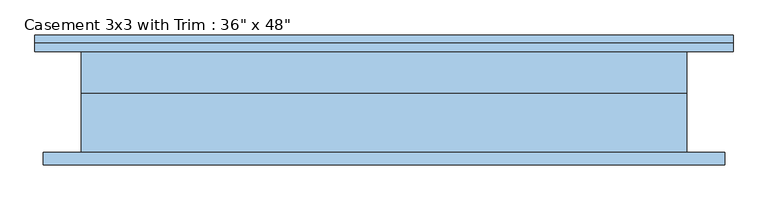
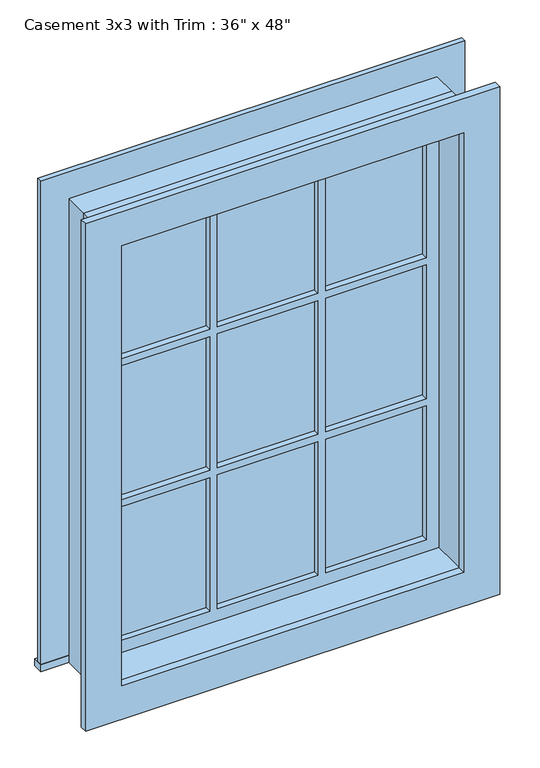
"""IFC4 building model written with IfcOpenShell, lengths in millimetres: window geometry."""

from ifc_helpers import new_model, si_unit, frame, origin, place, context, project, spatial, polyline, outline, extrude, source, transform, mapped, element, save


def window_d6f340c1(model_context):
    return source(origin(), model_context, "Body", "SweptSolid", [
        extrude(outline(polyline([(-527.05, 101.6), (527.05, 101.6), (527.05, 76.2), (-527.05, 76.2), (-527.05, 101.6)])), frame((0.0, 0.0, 1219.2), z_axis=(0.0, 0.0, 1.0), x_axis=(1.0, 0.0, 0.0)), (0.0, 0.0, 1.0), 19.05),
        extrude(outline(polyline([(2419.35, -438.15), (2419.35, 438.15), (1238.25, 438.15), (1238.25, 527.05), (2508.25, 527.05), (2508.25, -527.05), (1238.25, -527.05), (1238.25, -438.15), (2419.35, -438.15)])), frame((0.0, 76.2, 0.0), z_axis=(0.0, 1.0, 0.0), x_axis=(0.0, 0.0, 1.0)), (0.0, 0.0, 1.0), 12.7),
        extrude(outline(polyline([(143.9333333, 41.275), (393.7, 41.275), (393.7, 28.575), (143.9333333, 28.575), (143.9333333, 41.275)])), frame((0.0, 0.0, 2023.5333333), z_axis=(0.0, 0.0, 1.0), x_axis=(1.0, 0.0, 0.0)), (0.0, 0.0, 1.0), 351.3666667),
        extrude(outline(polyline([(-124.8833333, 41.275), (124.8833333, 41.275), (124.8833333, 28.575), (-124.8833333, 28.575), (-124.8833333, 41.275)])), frame((0.0, 0.0, 2023.5333333), z_axis=(0.0, 0.0, 1.0), x_axis=(1.0, 0.0, 0.0)), (0.0, 0.0, 1.0), 351.3666667),
        extrude(outline(polyline([(-393.7, 41.275), (-143.9333333, 41.275), (-143.9333333, 28.575), (-393.7, 28.575), (-393.7, 41.275)])), frame((0.0, 0.0, 2023.5333333), z_axis=(0.0, 0.0, 1.0), x_axis=(1.0, 0.0, 0.0)), (0.0, 0.0, 1.0), 351.3666667),
        extrude(outline(polyline([(-393.7, 41.275), (-143.9333333, 41.275), (-143.9333333, 28.575), (-393.7, 28.575), (-393.7, 41.275)])), frame((0.0, 0.0, 1653.1166667), z_axis=(0.0, 0.0, 1.0), x_axis=(1.0, 0.0, 0.0)), (0.0, 0.0, 1.0), 351.3666667),
        extrude(outline(polyline([(-124.8833333, 41.275), (124.8833333, 41.275), (124.8833333, 28.575), (-124.8833333, 28.575), (-124.8833333, 41.275)])), frame((0.0, 0.0, 1653.1166667), z_axis=(0.0, 0.0, 1.0), x_axis=(1.0, 0.0, 0.0)), (0.0, 0.0, 1.0), 351.3666667),
        extrude(outline(polyline([(143.9333333, 41.275), (393.7, 41.275), (393.7, 28.575), (143.9333333, 28.575), (143.9333333, 41.275)])), frame((0.0, 0.0, 1653.1166667), z_axis=(0.0, 0.0, 1.0), x_axis=(1.0, 0.0, 0.0)), (0.0, 0.0, 1.0), 351.3666667),
        extrude(outline(polyline([(143.9333333, 41.275), (393.7, 41.275), (393.7, 28.575), (143.9333333, 28.575), (143.9333333, 41.275)])), frame((0.0, 0.0, 1282.7), z_axis=(0.0, 0.0, 1.0), x_axis=(1.0, 0.0, 0.0)), (0.0, 0.0, 1.0), 351.3666667),
        extrude(outline(polyline([(-124.8833333, 41.275), (124.8833333, 41.275), (124.8833333, 28.575), (-124.8833333, 28.575), (-124.8833333, 41.275)])), frame((0.0, 0.0, 1282.7), z_axis=(0.0, 0.0, 1.0), x_axis=(1.0, 0.0, 0.0)), (0.0, 0.0, 1.0), 351.3666667),
        extrude(outline(polyline([(-393.7, 41.275), (-143.9333333, 41.275), (-143.9333333, 28.575), (-393.7, 28.575), (-393.7, 41.275)])), frame((0.0, 0.0, 1282.7), z_axis=(0.0, 0.0, 1.0), x_axis=(1.0, 0.0, 0.0)), (0.0, 0.0, 1.0), 351.3666667),
        extrude(outline(polyline([(2495.55, 514.35), (2495.55, -514.35), (1162.05, -514.35), (1162.05, 514.35), (2495.55, 514.35)]), holes=[polyline([(2406.65, 425.45), (1250.95, 425.45), (1250.95, -425.45), (2406.65, -425.45), (2406.65, 425.45)])]), frame((0.0, -95.25, 0.0), z_axis=(0.0, 1.0, 0.0), x_axis=(0.0, 0.0, 1.0)), (0.0, 0.0, 1.0), 19.05),
        extrude(outline(polyline([(2419.35, -438.15), (1238.25, -438.15), (1238.25, 438.15), (2419.35, 438.15), (2419.35, -438.15)]), holes=[polyline([(2374.9, -143.9333333), (2023.5333333, -143.9333333), (2023.5333333, -393.7), (2374.9, -393.7), (2374.9, -143.9333333)]), polyline([(2004.4833333, -143.9333333), (1653.1166667, -143.9333333), (1653.1166667, -393.7), (2004.4833333, -393.7), (2004.4833333, -143.9333333)]), polyline([(1634.0666667, -143.9333333), (1282.7, -143.9333333), (1282.7, -393.7), (1634.0666667, -393.7), (1634.0666667, -143.9333333)]), polyline([(2374.9, 124.8833333), (2023.5333333, 124.8833333), (2023.5333333, -124.8833333), (2374.9, -124.8833333), (2374.9, 124.8833333)]), polyline([(2004.4833333, 124.8833333), (1653.1166667, 124.8833333), (1653.1166667, -124.8833333), (2004.4833333, -124.8833333), (2004.4833333, 124.8833333)]), polyline([(1634.0666667, 124.8833333), (1282.7, 124.8833333), (1282.7, -124.8833333), (1634.0666667, -124.8833333), (1634.0666667, 124.8833333)]), polyline([(2374.9, 393.7), (2023.5333333, 393.7), (2023.5333333, 143.9333333), (2374.9, 143.9333333), (2374.9, 393.7)]), polyline([(2004.4833333, 393.7), (1653.1166667, 393.7), (1653.1166667, 143.9333333), (2004.4833333, 143.9333333), (2004.4833333, 393.7)]), polyline([(1634.0666667, 393.7), (1282.7, 393.7), (1282.7, 143.9333333), (1634.0666667, 143.9333333), (1634.0666667, 393.7)])]), frame((0.0, 12.7, 0.0), z_axis=(0.0, 1.0, 0.0), x_axis=(0.0, 0.0, 1.0)), (0.0, 0.0, 1.0), 44.45),
        extrude(outline(polyline([(2438.4, -457.2), (1219.2, -457.2), (1219.2, 457.2), (2438.4, 457.2), (2438.4, -457.2)]), holes=[polyline([(2406.65, -425.45), (2406.65, 425.45), (1250.95, 425.45), (1250.95, -425.45), (2406.65, -425.45)])]), frame((0.0, -76.2, 0.0), z_axis=(0.0, 1.0, 0.0), x_axis=(0.0, 0.0, 1.0)), (0.0, 0.0, 1.0), 88.9),
        extrude(outline(polyline([(2438.4, 457.2), (2438.4, -457.2), (1219.2, -457.2), (1219.2, 457.2), (2438.4, 457.2)]), holes=[polyline([(2419.35, 438.15), (1238.25, 438.15), (1238.25, -438.15), (2419.35, -438.15), (2419.35, 438.15)])]), frame((0.0, 12.7, 0.0), z_axis=(0.0, 1.0, 0.0), x_axis=(0.0, 0.0, 1.0)), (0.0, 0.0, 1.0), 63.5),
    ])


if __name__ == "__main__":
    model = new_model("IFC4")
    model_context = context("Model", 3, world=origin())
    ifc_project = project(units=[si_unit("LENGTHUNIT", "METRE", prefix="MILLI")], contexts=[model_context])
    site = spatial("IfcSite", under=ifc_project)
    building = spatial("IfcBuilding", under=site)
    placement = place(None, origin())
    window_shape = window_d6f340c1(model_context)
    element("IfcWindow", 1, ObjectType="Casement 3x3 with Trim : 36\" x 48\"", at=placement, inside=building, context=model_context, shape_type="MappedRepresentation", body=[
        mapped(window_shape, transform((0.0, 0.0, 0.0), x_axis=(1.0, 0.0, 0.0), y_axis=(0.0, 1.0, 0.0), z_axis=(0.0, 0.0, 1.0))),
    ])
    save(model, "model.ifc")

# Revit data of these elements
# Type "Casement 3x3 with Trim : 36\" x 48\""
#   Type Mark = "10"
#   Construction Type Id = "GSP4R"
#   Assembly Code = "B2020100"
#   Analytic Construction = "1/8 in Pilkington single glazing"
#   Visual Light Transmittance = 0.9
#   Solar Heat Gain Coefficient = 0.78
#   Heat Transfer Coefficient (U) = 0.6496 BTU/(h·ft²·°F)
#   Height = 4' - 0"
#   Default Sill Height = 4' - 0"
#   Trim Projection - Ext. = 0' - 0 1/2"
#   Trim Projection - Int. = 0' - 0 3/4"
#   Trim Width - Exterior = 0' - 3 1/2"
#   Trim Width - Interior = 0' - 3 1/2"
#   Width = 3' - 0"
#   Window Inset = 0' - 0 3/4"
#   Define Thermal Properties by = 1
#   Glass Pane Material = Glass
#   Sash Material = Sash
#   Trim Exterior Material = Trim
#   Trim Interior Material = Trim
#   Wall Closure = (empty or 0)
# Element 1 (IfcWindow, "Casement 3x3 with Trim : 36\" x 48\"")
#   Materials on its faces: "Sash", "Glass", "Trim"
# Materials
#   "Glass": class "Glass", colour RGB 0 128 192, transparency 0.75, Description = "Soda Lime Glass", Cost = 0
#   "Sash": class "Wood", colour RGB 224 178 126, transparency 0
#   "Trim": class "Wood", colour RGB 224 178 126, transparency 0
